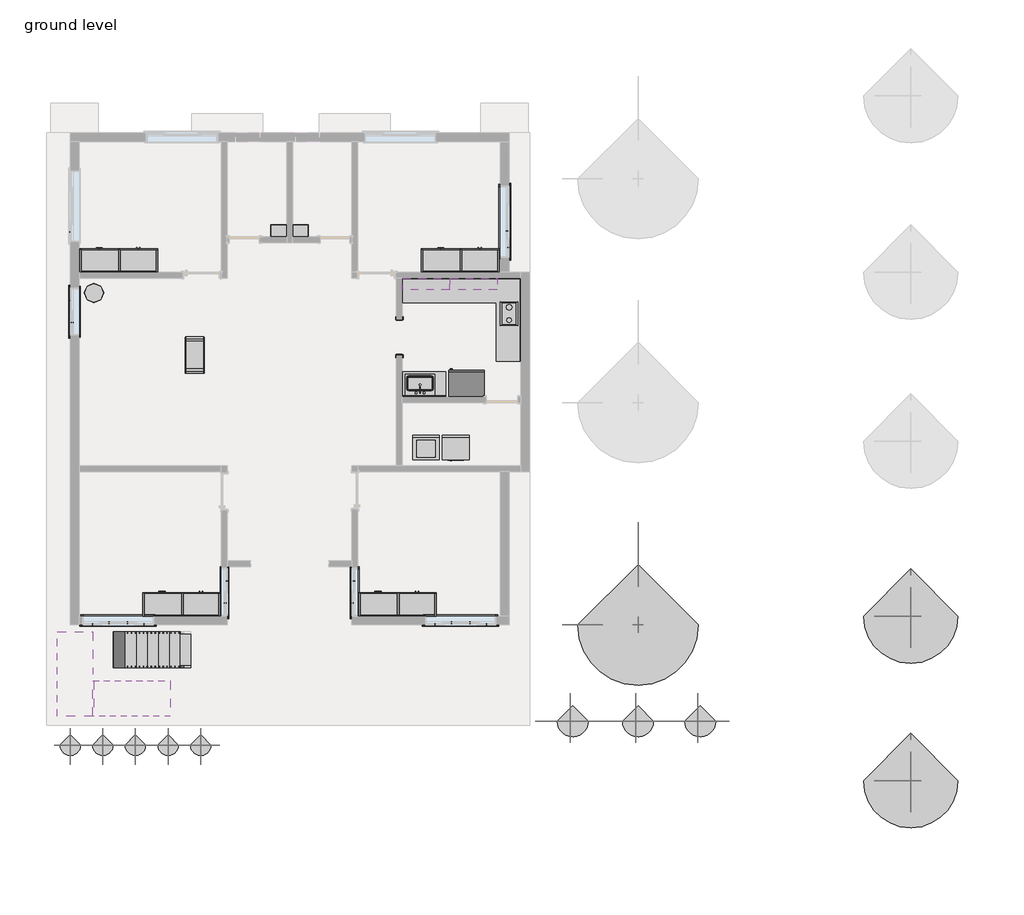
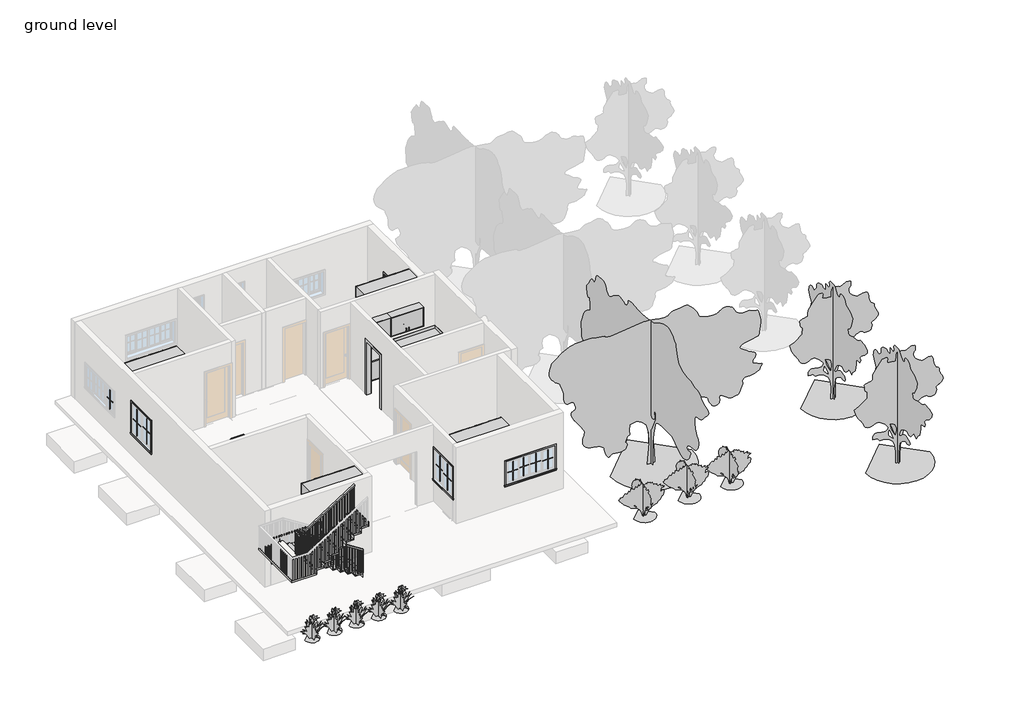
# One storey, part 3 of 4: 33 proxies, 15 furniture elements, 11 geographic elements, 3 flow terminals, 2 stair flights, 1 railing, 1 slab.
# Revit data of these elements (continued)
# Type "RPC Plant - Tropical" (continued)
#   built-in parameter 1005198 = "{2, 15},{39, RPC-16-FWM5-GM7X-C67P-4000-ST1L-LVER-AU},{1, 0},{1, 0},{2, 35},{1, 8},{5, Color},{1, 0},{1, 0},{3, 0.8},{3, 0.8},{3, 0.8},{1, 8},{7, BBoxMin},{1, 0},{1, 0},{1, 0},{1, 0},{1, 0},{1, 8},{7, BBoxMax},{1, 0},{1, 0},{1, 0},{1, 0},{1, 0},{2, 11},{9, RPCTypeId},{1, 0},{1, 0},{39, RPC-16-FWM5-GM7X-C67P-4000-ST1L-LVER-AU},{1, 6},{14, RPCPlantHeight},{1, 0},{1, 0},{1, 3},{2, 11},{7, keyword},{1, 0},{1, 0},{99, :Geometry:RPC:Crane Lily:strelitzia:reinae:crane lily:plants:shrub:flower:tropical:bird-of-paradise},{2, 11},{8, category},{1, 0},{1, 0},{17, :Shrubs [General]},{2, 11},{12, LocalizedUID},{1, 0},{1, 0},{10, Crane Lily},{2, 14},{6, Height},{1, 0},{1, 0},{1, 3},{1, 2},{16, Cast Reflections},{1, 0},{1, 0},{1, 0},{1, 2},{12, Cast Shadows},{1, 0},{1, 0},{1, 1},{1, 2},{9, Lock View},{1, 0},{1, 0},{1, 0},{1, 4},{5, ViewC},{1, 0},{1, 0},{1, 0},{2, 11},{20, AdvancedUIDefinition},{1, 0},{1, 0},{0, },{2, 11},{10, AssetLibID},{1, 0},{1, 0},{36, 4D3F6E72-3F99-4203-98E9-AF80B3C7A7A4},{2, 11},{10, BaseSchema},{1, 0},{1, 0},{9, RPCSchema},{2, 11},{12, ExchangeGUID},{1, 0},{1, 0},{0, },{1, 2},{6, Hidden},{1, 0},{1, 0},{1, 0},{1, 4},{11, RPCCategory},{1, 0},{1, 0},{1, 0},{2, 11},{8, RPCImage},{1, 0},{1, 0},{0, },{1, 4},{13, SchemaVersion},{1, 0},{1, 0},{1, 4},{2, 11},{12, UIDefinition},{1, 0},{1, 0},{0, },{2, 11},{6, UIName},{1, 0},{1, 0},{39, RPC-16-FWM5-GM7X-C67P-4000-ST1L-LVER-AU},{2, 11},{11, VersionGUID},{1, 0},{1, 0},{9, RPCSchema},{2, 11},{9, assettype},{1, 0},{1, 0},{11, RPCGeometry},{2, 11},{11, description},{1, 0},{1, 0},{0, },{2, 11},{9, localname},{1, 0},{1, 0},{3, RPC},{2, 11},{9, localtype},{1, 0},{1, 0},{3, RPC},{1, 4},{8, revision},{1, 0},{1, 0},{1, 1},{2, 11},{9, thumbnail},{1, 0},{1, 0},{0, },{1, 4},{7, version},{1, 0},{1, 0},{1, 1},{1, 2},{20, RPC_Cast Reflections},{1, 0},{1, 0},{1, 1},{1, 2},{16, RPC_Cast Shadows},{1, 0},{1, 0},{1, 1},{1, 2},{13, RPC_Lock View},{1, 0},{1, 0},{1, 0},{1, 4},{9, RPC_ViewC},{1, 0},{1, 0},{1, 0},{21, assetlibrary_base.fbx},{1, 5},"
#   built-in parameter 1005195 = "RPC-16-FWM5-GM7X-C67P-4000-ST1L-LVER-AU"
#   Assembly Code = "G2050500"
#   Height = 3' - 0"
#   Default Elevation = 0
# Type "RPC Plant - Tropical"
#   built-in parameter 1005198 = "{2, 15},{39, RPC-16-G3GK-N2Q0-PN0G-6000-ST1L-LVER-AU},{1, 0},{1, 0},{2, 35},{1, 8},{5, Color},{1, 0},{1, 0},{3, 0.8},{3, 0.8},{3, 0.8},{1, 8},{7, BBoxMin},{1, 0},{1, 0},{1, 0},{1, 0},{1, 0},{1, 8},{7, BBoxMax},{1, 0},{1, 0},{1, 0},{1, 0},{1, 0},{2, 11},{9, RPCTypeId},{1, 0},{1, 0},{39, RPC-16-G3GK-N2Q0-PN0G-6000-ST1L-LVER-AU},{1, 6},{14, RPCPlantHeight},{1, 0},{1, 0},{3, 4.5},{2, 11},{7, keyword},{1, 0},{1, 0},{80, :Geometry:RPC:Honey Myrtle:honey myrtle:melaleuca spathulata:tropical:austrailia},{2, 11},{8, category},{1, 0},{1, 0},{17, :Shrubs [General]},{2, 11},{12, LocalizedUID},{1, 0},{1, 0},{12, Honey Myrtle},{2, 14},{6, Height},{1, 0},{1, 0},{3, 4.5},{1, 2},{16, Cast Reflections},{1, 0},{1, 0},{1, 0},{1, 2},{12, Cast Shadows},{1, 0},{1, 0},{1, 1},{1, 2},{9, Lock View},{1, 0},{1, 0},{1, 0},{1, 4},{5, ViewC},{1, 0},{1, 0},{1, 0},{2, 11},{20, AdvancedUIDefinition},{1, 0},{1, 0},{0, },{2, 11},{10, AssetLibID},{1, 0},{1, 0},{36, 4D3F6E72-3F99-4203-98E9-AF80B3C7A7A4},{2, 11},{10, BaseSchema},{1, 0},{1, 0},{9, RPCSchema},{2, 11},{12, ExchangeGUID},{1, 0},{1, 0},{0, },{1, 2},{6, Hidden},{1, 0},{1, 0},{1, 0},{1, 4},{11, RPCCategory},{1, 0},{1, 0},{1, 0},{2, 11},{8, RPCImage},{1, 0},{1, 0},{0, },{1, 4},{13, SchemaVersion},{1, 0},{1, 0},{1, 4},{2, 11},{12, UIDefinition},{1, 0},{1, 0},{0, },{2, 11},{6, UIName},{1, 0},{1, 0},{39, RPC-16-G3GK-N2Q0-PN0G-6000-ST1L-LVER-AU},{2, 11},{11, VersionGUID},{1, 0},{1, 0},{9, RPCSchema},{2, 11},{9, assettype},{1, 0},{1, 0},{11, RPCGeometry},{2, 11},{11, description},{1, 0},{1, 0},{0, },{2, 11},{9, localname},{1, 0},{1, 0},{3, RPC},{2, 11},{9, localtype},{1, 0},{1, 0},{3, RPC},{1, 4},{8, revision},{1, 0},{1, 0},{1, 1},{2, 11},{9, thumbnail},{1, 0},{1, 0},{0, },{1, 4},{7, version},{1, 0},{1, 0},{1, 1},{1, 2},{20, RPC_Cast Reflections},{1, 0},{1, 0},{1, 1},{1, 2},{16, RPC_Cast Shadows},{1, 0},{1, 0},{1, 1},{1, 2},{13, RPC_Lock View},{1, 0},{1, 0},{1, 0},{1, 4},{9, RPC_ViewC},{1, 0},{1, 0},{1, 0},{21, assetlibrary_base.fbx},{1, 5},"
#   built-in parameter 1005195 = "RPC-16-G3GK-N2Q0-PN0G-6000-ST1L-LVER-AU"
#   Assembly Code = "G2050500"
#   Height = 4' - 6"
#   Default Elevation = 0
# Type "RPC Tree - Deciduous : Common Apple - 20'"
#   built-in parameter 1005198 = "{2, 15},{39, RPC-16-FXGK-4KXX-PJE5-6000-ST1L-LVER-AU},{1, 0},{1, 0},{2, 35},{1, 8},{5, Color},{1, 0},{1, 0},{3, 0.8},{3, 0.8},{3, 0.8},{1, 8},{7, BBoxMin},{1, 0},{1, 0},{1, 0},{1, 0},{1, 0},{1, 8},{7, BBoxMax},{1, 0},{1, 0},{1, 0},{1, 0},{1, 0},{2, 11},{9, RPCTypeId},{1, 0},{1, 0},{39, RPC-16-FXGK-4KXX-PJE5-6000-ST1L-LVER-AU},{1, 6},{14, RPCPlantHeight},{1, 0},{1, 0},{2, 20},{2, 11},{7, keyword},{1, 0},{1, 0},{168, :Geometry:RPC:Common Apple:Malus sylvestris:occurs in southern Ontario near Lakes Erie and Ontario.  Numerous cultivars planted in orchards; naturalized in many places.},{2, 11},{8, category},{1, 0},{1, 0},{16, :Trees [General]},{2, 11},{12, LocalizedUID},{1, 0},{1, 0},{12, Common Apple},{2, 14},{6, Height},{1, 0},{1, 0},{2, 20},{1, 2},{16, Cast Reflections},{1, 0},{1, 0},{1, 0},{1, 2},{12, Cast Shadows},{1, 0},{1, 0},{1, 1},{1, 2},{9, Lock View},{1, 0},{1, 0},{1, 0},{1, 4},{5, ViewC},{1, 0},{1, 0},{1, 0},{2, 11},{20, AdvancedUIDefinition},{1, 0},{1, 0},{0, },{2, 11},{10, AssetLibID},{1, 0},{1, 0},{36, 4D3F6E72-3F99-4203-98E9-AF80B3C7A7A4},{2, 11},{10, BaseSchema},{1, 0},{1, 0},{9, RPCSchema},{2, 11},{12, ExchangeGUID},{1, 0},{1, 0},{0, },{1, 2},{6, Hidden},{1, 0},{1, 0},{1, 0},{1, 4},{11, RPCCategory},{1, 0},{1, 0},{1, 0},{2, 11},{8, RPCImage},{1, 0},{1, 0},{0, },{1, 4},{13, SchemaVersion},{1, 0},{1, 0},{1, 4},{2, 11},{12, UIDefinition},{1, 0},{1, 0},{0, },{2, 11},{6, UIName},{1, 0},{1, 0},{39, RPC-16-FXGK-4KXX-PJE5-6000-ST1L-LVER-AU},{2, 11},{11, VersionGUID},{1, 0},{1, 0},{9, RPCSchema},{2, 11},{9, assettype},{1, 0},{1, 0},{11, RPCGeometry},{2, 11},{11, description},{1, 0},{1, 0},{0, },{2, 11},{9, localname},{1, 0},{1, 0},{3, RPC},{2, 11},{9, localtype},{1, 0},{1, 0},{3, RPC},{1, 4},{8, revision},{1, 0},{1, 0},{1, 1},{2, 11},{9, thumbnail},{1, 0},{1, 0},{0, },{1, 4},{7, version},{1, 0},{1, 0},{1, 1},{1, 2},{20, RPC_Cast Reflections},{1, 0},{1, 0},{1, 1},{1, 2},{16, RPC_Cast Shadows},{1, 0},{1, 0},{1, 1},{1, 2},{13, RPC_Lock View},{1, 0},{1, 0},{1, 0},{1, 4},{9, RPC_ViewC},{1, 0},{1, 0},{1, 0},{21, assetlibrary_base.fbx},{1, 5},"
#   built-in parameter 1005195 = "RPC-16-FXGK-4KXX-PJE5-6000-ST1L-LVER-AU"
#   Type Comments = "Common Apple"
#   Assembly Code = "G2050500"
#   Height = 20' - 0"
#   Default Elevation = 0
# Type "RPC Tree - Deciduous : Japanese Cherry - 15'"
#   built-in parameter 1005198 = "{2, 15},{39, RPC-16-FXGW-2MQ0-PN7K-A000-ST1L-LVER-AU},{1, 0},{1, 0},{2, 35},{1, 8},{5, Color},{1, 0},{1, 0},{3, 0.8},{3, 0.8},{3, 0.8},{1, 8},{7, BBoxMin},{1, 0},{1, 0},{1, 0},{1, 0},{1, 0},{1, 8},{7, BBoxMax},{1, 0},{1, 0},{1, 0},{1, 0},{1, 0},{2, 11},{9, RPCTypeId},{1, 0},{1, 0},{39, RPC-16-FXGW-2MQ0-PN7K-A000-ST1L-LVER-AU},{1, 6},{14, RPCPlantHeight},{1, 0},{1, 0},{2, 15},{2, 11},{7, keyword},{1, 0},{1, 0},{207, :Geometry:RPC:Japanese Flowering Cherry:Prunus serrulata Lindl:A landscape tree:valued for its abundant showy flowers; native to China and Japan.  Hardy only in the mildest parts of Canada and farther south.},{2, 11},{8, category},{1, 0},{1, 0},{16, :Trees [General]},{2, 11},{12, LocalizedUID},{1, 0},{1, 0},{25, Japanese Flowering Cherry},{2, 14},{6, Height},{1, 0},{1, 0},{2, 15},{1, 2},{16, Cast Reflections},{1, 0},{1, 0},{1, 0},{1, 2},{12, Cast Shadows},{1, 0},{1, 0},{1, 1},{1, 2},{9, Lock View},{1, 0},{1, 0},{1, 0},{1, 4},{5, ViewC},{1, 0},{1, 0},{1, 0},{2, 11},{20, AdvancedUIDefinition},{1, 0},{1, 0},{0, },{2, 11},{10, AssetLibID},{1, 0},{1, 0},{36, 4D3F6E72-3F99-4203-98E9-AF80B3C7A7A4},{2, 11},{10, BaseSchema},{1, 0},{1, 0},{9, RPCSchema},{2, 11},{12, ExchangeGUID},{1, 0},{1, 0},{0, },{1, 2},{6, Hidden},{1, 0},{1, 0},{1, 0},{1, 4},{11, RPCCategory},{1, 0},{1, 0},{1, 0},{2, 11},{8, RPCImage},{1, 0},{1, 0},{0, },{1, 4},{13, SchemaVersion},{1, 0},{1, 0},{1, 4},{2, 11},{12, UIDefinition},{1, 0},{1, 0},{0, },{2, 11},{6, UIName},{1, 0},{1, 0},{39, RPC-16-FXGW-2MQ0-PN7K-A000-ST1L-LVER-AU},{2, 11},{11, VersionGUID},{1, 0},{1, 0},{9, RPCSchema},{2, 11},{9, assettype},{1, 0},{1, 0},{11, RPCGeometry},{2, 11},{11, description},{1, 0},{1, 0},{0, },{2, 11},{9, localname},{1, 0},{1, 0},{3, RPC},{2, 11},{9, localtype},{1, 0},{1, 0},{3, RPC},{1, 4},{8, revision},{1, 0},{1, 0},{1, 1},{2, 11},{9, thumbnail},{1, 0},{1, 0},{0, },{1, 4},{7, version},{1, 0},{1, 0},{1, 1},{1, 2},{20, RPC_Cast Reflections},{1, 0},{1, 0},{1, 1},{1, 2},{16, RPC_Cast Shadows},{1, 0},{1, 0},{1, 1},{1, 2},{13, RPC_Lock View},{1, 0},{1, 0},{1, 0},{1, 4},{9, RPC_ViewC},{1, 0},{1, 0},{1, 0},{21, assetlibrary_base.fbx},{1, 5},"
#   built-in parameter 1005195 = "RPC-16-FXGW-2MQ0-PN7K-A000-ST1L-LVER-AU"
#   Type Comments = "Japanese Cherry"
#   Assembly Code = "G2050500"
#   Height = 15' - 0"
#   Default Elevation = 0
# Type "Handrail - Rectangular"
#   Assembly Code = "C2010400"
#   built-in parameter 1008612 = 0.0416667 (stored number, unit not read)
#   built-in parameter 1008611 = 0.0416667 (stored number, unit not read)
#   built-in parameter 1008609 = 0.333333 (stored number, unit not read)
#   built-in parameter 1008604 = 0.166667 (stored number, unit not read)
#   built-in parameter 1008603 = 0.166667 (stored number, unit not read)
#   Railing Height = 3' - 0"
#   built-in parameter 1008630 = 2
#   built-in parameter 1008610 = 2
#   built-in parameter 1008618 = Baluster - Square : 3/4"
# Element 1 (IfcBuildingElementProxy, "Cook Top-2 Unit : 12\" x 18\" 2")
#   Phase Created = New Construction
#   Materials on its faces: "Metal - Steel, Polished", "Metal - Chrome"
# Element 2 (IfcBuildingElementProxy, "Dryer : 27\" x 25\" x 35\"")
#   Phase Created = New Construction
#   Materials on its faces: "Metal - Paint Finish - Ivory,Glossy"
# Elements 3, 4, 5, 6, 7, 8 (IfcBuildingElementProxy, "Muntin Pattern_2x2 : Muntin Pattern_2x2")
#   Width = 1' - 8 5/8"
#   Height = 3' - 6 1/4"
#   Interior Material = Wood - Stained
#   Exterior Material = Clad - White
#   Phase Created = New Construction
#   Materials on its faces: "Clad - White", "Wood - Stained"
# Elements 9, 10, 11, 12, 13, 14, 15, 16, 17, 18, 19 (IfcBuildingElementProxy, "Muntin Pattern_2x2 : Muntin Pattern_2x2")
#   Width = 1' - 3"
#   Height = 2' - 6 1/4"
#   Interior Material = Wood - Stained
#   Exterior Material = Clad - White
#   Phase Created = New Construction
#   Materials on its faces: "Clad - White", "Wood - Stained"
# Element 20 (IfcBuildingElementProxy, "Passage Opening-Cased : 36\" x 84\"")
#   Phase Created = New Construction
#   Materials on its faces: "Door - Frame"
# Elements 21, 22, 23 (IfcBuildingElementProxy, "Trim-Window-Exterior-Flat : with Sill")
#   Opening Width = 4' - 0"
#   Opening Height = 4' - 0"
#   Trim Material = Clad - White
#   Phase Created = New Construction
#   Materials on its faces: "Clad - White"
# Elements 24, 25, 26 (IfcBuildingElementProxy, "Trim-Window-Exterior-Flat : with Sill")
#   Opening Width = 6' - 0"
#   Opening Height = 3' - 0"
#   Trim Material = Clad - White
#   Phase Created = New Construction
#   Materials on its faces: "Clad - White"
# Elements 27, 28, 29 (IfcBuildingElementProxy, "Trim-Window-Interior-Flat : Picture Frame")
#   Opening Width = 4' - 0"
#   Opening Height = 4' - 0"
#   Trim Material = Wood - Stained
#   Phase Created = New Construction
#   Materials on its faces: "Wood - Stained"
# Elements 30, 31, 32 (IfcBuildingElementProxy, "Trim-Window-Interior-Flat : Picture Frame")
#   Opening Width = 6' - 0"
#   Opening Height = 3' - 0"
#   Trim Material = Wood - Stained
#   Phase Created = New Construction
#   Materials on its faces: "Wood - Stained"
# Element 33 (IfcBuildingElementProxy, "Washer : 27\" x 25\" x 35\"")
#   Phase Created = New Construction
#   Materials on its faces: "Metal - Paint Finish - Ivory,Matte"
# Element 34 (IfcFlowTerminal, "Sink - Work : 20\"x18\" 2")
#   Mark = "7"
#   Flow Pressure = 8.00 psi
#   Phase Created = New Construction
# Element 35 (IfcFlowTerminal, "Sink - Work : 20\"x18\" 2")
#   Mark = "9"
#   Flow Pressure = 8.00 psi
#   Phase Created = New Construction
# Element 36 (IfcFlowTerminal, "Sink Kitchen-Single : 30\" x 21\"")
#   Mark = "5"
#   Phase Created = New Construction
#   Materials on its faces: "Steel, Polished"
# Element 37 (IfcFurniture)
#   Phase Created = New Construction
# Element 38 (IfcFurniture)
#   Phase Created = New Construction
#   Materials on its faces: "Default", "Default 3", "Default 2"
# Elements 39, 40, 41, 42 (IfcFurniture, "1Wardrobe_6271 : 1Wardrobe_6271")
#   Phase Created = New Construction
#   Materials on its faces: "Phase - Demo", "Default Wall", "Phase - Exist", "Default"
# Element 43 (IfcFurniture, "48\" 2")
#   Phase Created = New Construction
#   Materials on its faces: "Cabinet", "Cabinets - Handles", "Cabinets"
# Element 44 (IfcFurniture, "48\" 3")
#   Phase Created = New Construction
#   Materials on its faces: "Cabinet", "Cabinets - Handles", "Cabinets"
# Element 45 (IfcFurniture, "Base Cabinet-Combo01 : 30\" 2")
#   Phase Created = New Construction
#   Materials on its faces: "Cabinet"
# Element 46 (IfcFurniture, "Base Cabinet-Corner Unit-Square : 36\"")
#   Phase Created = New Construction
#   Materials on its faces: "Cabinets", "Cabinets - Handles"
# Element 47 (IfcFurniture, "Counter Top w Sink Hole : 24\" Depth")
#   Sink Opening Width = 2' - 3"
#   Sink Opening Depth = 1' - 3"
#   Sink Location To Wall = 0' - 6"
#   Sink Location = 2' - 2"
#   Length = 3' - 8"
#   Phase Created = New Construction
#   Materials on its faces: "Counter Top"
# Element 48 (IfcFurniture, "Counter Top-L Shaped : 24\" Depth")
#   Length - Leg 2 = 10' - 0"
#   Length - Leg 1 = 7' - 0"
#   Phase Created = New Construction
#   Materials on its faces: "Counter Top"
# Element 49 (IfcFurniture, "Table-Trio End : 20\" Diameter")
#   Phase Created = New Construction
#   Materials on its faces: "Wood - Birch", "Laminate - Ivory,Matte"
# Elements 50, 51 (IfcFurniture, "Upper Cabinet-Pass-Thru : 48\" x 30\" x 12\"")
#   Phase Created = New Construction
#   Materials on its faces: "Cabinet"
# Elements 52, 53, 54, 55, 56, 57, 58, 59 (IfcGeographicElement, "RPC Plant - Tropical")
#   Phase Created = New Construction
# Element 60 (IfcGeographicElement, "RPC Tree - Deciduous : Common Apple - 20'")
#   Phase Created = New Construction
# Elements 61, 62 (IfcGeographicElement, "RPC Tree - Deciduous : Japanese Cherry - 15'")
#   Phase Created = New Construction
# Element 63 (IfcRailing, "Handrail - Rectangular")
#   Phase Created = New Construction
# Element 64 (IfcSlab, "Non-Monolithic Landing")
#   Phase Created = New Construction
# Elements 65, 66 (IfcStairFlight, "2\" Tread 1\" Nosing 1/4\" Riser")
#   Phase Created = New Construction
# Materials
#   "Metal - Chrome": colour RGB 17 17 17, transparency 0
#   "Metal - Steel, Polished": colour RGB 57 57 57, transparency 0
#   "Metal - Paint Finish - Ivory,Glossy": colour RGB 247 247 239, transparency 0
#   "Door - Frame": colour RGB 118 70 51, transparency 0, Cost = 0
#   "Metal - Paint Finish - Ivory,Matte": colour RGB 247 247 239, transparency 0
#   "Steel, Polished": class "Metal", colour RGB 192 192 192, transparency 0, Description = "Polished steel", Cost = 0
#   "Cabinets - Handles": colour RGB 57 57 57, transparency 0
#   "Cabinets": colour RGB 249 249 249, transparency 0
#   "Wood - Birch": colour RGB 230 196 162, transparency 0
#   "Laminate - Ivory,Matte": colour RGB 127 127 127, transparency 0
#   "Clad - White": class "Wood", colour RGB 242 242 238, transparency 0, Cost = 0
#   "Wood - Stained": class "Wood", colour RGB 224 178 126, transparency 0, Cost = 0
#   "Default": colour RGB 127 127 127, transparency 0, Cost = 0
#   "Default 3": class "Glass", colour RGB 127 127 127, transparency 0
#   "Default 2": class "Plastic", colour RGB 127 127 127, transparency 0
#   "Phase - Demo": class "System", colour RGB 255 0 0, transparency 0.4, Cost = 0
#   "Default Wall": colour RGB 128 128 128, transparency 0, Cost = 0
#   "Phase - Exist": class "System", colour RGB 127 127 127, transparency 0, Cost = 0
#   "Cabinet": colour RGB 204 122 2, transparency 0
#   "Counter Top": class "Wood", colour RGB 226 177 128, transparency 0
